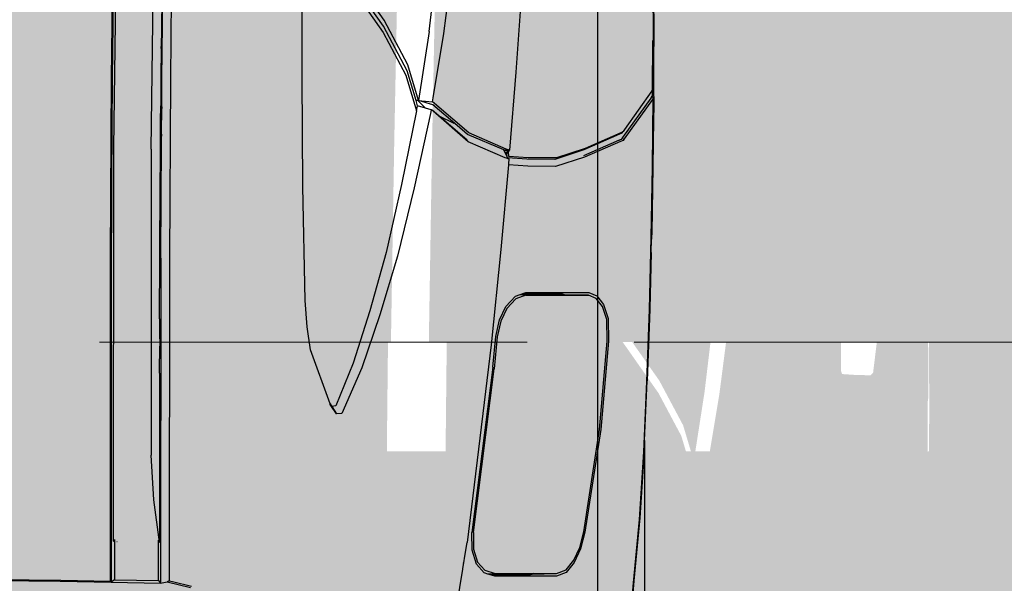
# Model space of a CAD drawing. Units: inches. Extents: x 1884 to 2398, y 474 to 1488.
# Tile 9 of 39: x 2247 to 2275, y 604 to 620. Entities that reach past the tile are written whole.
import ezdxf

# ---------------------------------------------------------------- set-up
doc = ezdxf.new("R2010")
doc.units = ezdxf.units.IN
doc.header["$MEASUREMENT"] = 0
doc.linetypes.add('ACAD_ISO02W100', pattern=[15, 12, -3])
doc.layers.get('0').update_dxf_attribs({"color": 250})
for name, color, linetype, lineweight in [('A-ANNO-DIMS', 2, 'Continuous', 18), ('A-FLOR-OVHD', 8, 'ACAD_ISO02W100', 18), ('C-VEHI', 8, 'Continuous', 18)]:
    doc.layers.add(name, color=color, linetype=linetype, lineweight=lineweight)
doc.layers.add('Edges', color=250, linetype='Continuous')
doc.layers.add('L-PVMT-PATT', color=9, linetype='Continuous', lineweight=13, true_color=0xc7c8ca)
doc.styles.get("Standard").update_dxf_attribs({"font": 'arial.ttf'})
doc.dimstyles.get("Standard").update_dxf_attribs({"dimtxt": 7, "dimasz": 0.18, "dimexe": 0.18, "dimexo": 0.0625, "dimgap": 0.09, "dimtad": 0, "dimtih": 1, "dimtoh": 1, "dimzin": 0, "dimdsep": 46, "dimlunit": 3, "dimtxsty": 'Standard', "dimcen": 0.09, "dimadec": 0, "dimazin": 0, "dimtfac": 1, "dimtofl": 0, "dimtmove": 0, "dimatfit": 3, "dimfxl": 1, "dimtolj": 1, "dimtzin": 0, "dimarcsym": 0})

# ---------------------------------------------------------------- blocks, each defined once
blk = doc.blocks.new('Nissan Qashqai pl')
at = {"layer": 'Edges'}
for p, q in [((10.61514, 12.81589), (10.66445, 12.81615)), ((10.61756, 12.81643), (10.66511, 12.81673)), ((10.66445, 12.81615), (10.7078, 12.81595)), ((10.66511, 12.81673), (10.66601, 12.81673)), ((10.66601, 12.81673), (10.67702, 12.8167)), ((10.67289, 12.81571), (10.70817, 12.81563)), ((10.68094, 12.81673), (10.67702, 12.8167)), ((10.71276, 12.81662), (10.68094, 12.81673)), ((10.7078, 12.81595), (10.70826, 12.81563)), ((10.70817, 12.81563), (10.7078, 12.81595)), ((10.70855, 12.81529), (10.70817, 12.81563)), ((10.70817, 12.81563), (10.70826, 12.81563)), ((10.70826, 12.81563), (10.70875, 12.81529)), ((10.70826, 12.81563), (10.71254, 12.81562)), ((10.70875, 12.81529), (10.7363, 12.79586)), ((10.71391, 12.81637), (10.71254, 12.81562)), ((10.71373, 12.81477), (10.71254, 12.81562)), ((10.71276, 12.81662), (10.76246, 12.8161)), ((10.71276, 12.81662), (10.72402, 12.81662)), ((10.71373, 12.81477), (10.71377, 12.81474)), ((10.74185, 12.79469), (10.71377, 12.81474)), ((10.71391, 12.81637), (10.7148, 12.81574)), ((10.76281, 12.81584), (10.71391, 12.81637)), ((10.7148, 12.81574), (10.74291, 12.79564)), ((10.76848, 12.8161), (10.72402, 12.81662)), ((10.76246, 12.8161), (10.76281, 12.8161)), ((10.76281, 12.8161), (10.80986, 12.81522)), ((10.81307, 12.81492), (10.76281, 12.81584)), ((10.76883, 12.8161), (10.76848, 12.8161)), ((10.80986, 12.81522), (10.76883, 12.8161)), ((10.80986, 12.81522), (10.81313, 12.81516)), ((10.86443, 12.81355), (10.81307, 12.81492)), ((10.81337, 12.81516), (10.81313, 12.81516)), ((10.81337, 12.81516), (10.81418, 12.81516)), ((10.81418, 12.81516), (10.81424, 12.81516)), ((10.82367, 12.81488), (10.81424, 12.81516)), ((10.82367, 12.81488), (10.86395, 12.8138)), ((10.85956, 12.81381), (10.85889, 12.81383)), ((10.86421, 12.81363), (10.85956, 12.81381)), ((10.86395, 12.8138), (10.8642, 12.81379)), ((10.8642, 12.81379), (10.91525, 12.81203)), ((10.91576, 12.81179), (10.86443, 12.81355)), ((10.95774, 12.81008), (10.91525, 12.81203)), ((10.9657, 12.8095), (10.91576, 12.81179)), ((10.95774, 12.81008), (10.9649, 12.80975)), ((10.95774, 12.81008), (11.12826, 12.81008)), ((10.9649, 12.80975), (11.01272, 12.8067)), ((11.01381, 12.80644), (10.9657, 12.8095)), ((11.01272, 12.8067), (11.05762, 12.80257)), ((11.05899, 12.80228), (11.01381, 12.80644)), ((11.05762, 12.80257), (11.07977, 12.80077)), ((11.07681, 12.80079), (11.05899, 12.80228)), ((10.7363, 12.79586), (10.73758, 12.79499)), ((10.73869, 12.794), (10.73758, 12.79499)), ((10.73758, 12.79499), (10.73776, 12.79462)), ((10.73776, 12.79462), (10.73792, 12.79451)), ((10.73776, 12.79462), (10.73846, 12.79316)), ((10.73846, 12.79316), (10.74965, 12.76789)), ((10.73869, 12.794), (10.73956, 12.79223)), ((10.73956, 12.79223), (10.7507, 12.76687)), ((10.74298, 12.79387), (10.74185, 12.79469)), ((10.74324, 12.79539), (10.74265, 12.7954)), ((10.74291, 12.79564), (10.74324, 12.79539)), ((10.74336, 12.79302), (10.74298, 12.79387)), ((10.74408, 12.79539), (10.74324, 12.79539)), ((10.74324, 12.79539), (10.74404, 12.7948)), ((10.74374, 12.79215), (10.74336, 12.79302)), ((10.74376, 12.7921), (10.74374, 12.79215)), ((10.74376, 12.7921), (10.75486, 12.76658)), ((10.74404, 12.7948), (10.74477, 12.79302)), ((10.74477, 12.79302), (10.75592, 12.76744)), ((10.86074, 12.78081), (10.87075, 12.78409)), ((10.87075, 12.78409), (10.88688, 12.78445)), ((10.88703, 12.78354), (10.87156, 12.78319)), ((10.88688, 12.78445), (10.94987, 12.77894)), ((10.94977, 12.77808), (10.88703, 12.78354)), ((10.85458, 12.77617), (10.86074, 12.78081)), ((10.86225, 12.78009), (10.85648, 12.77573)), ((10.87156, 12.78319), (10.86225, 12.78009)), ((11.02261, 12.76681), (10.94977, 12.77808)), ((10.94987, 12.77894), (11.02295, 12.7676)), ((10.85228, 12.77036), (10.85458, 12.77617)), ((10.85228, 12.72552), (10.85228, 12.77036)), ((10.85427, 12.77015), (10.85384, 12.753)), ((10.85648, 12.77573), (10.85427, 12.77015)), ((10.85427, 12.72549), (10.85427, 12.77015)), ((10.74965, 12.76789), (10.75648, 12.74726)), ((10.7507, 12.76687), (10.75747, 12.74624)), ((10.75592, 12.76744), (10.76258, 12.74675)), ((11.03387, 12.76392), (11.02261, 12.76681)), ((11.02295, 12.7676), (11.03477, 12.76454)), ((11.04293, 12.75972), (11.03387, 12.76392)), ((11.03477, 12.76454), (11.04442, 12.76006)), ((11.04973, 12.75421), (11.04293, 12.75972)), ((11.04442, 12.76006), (11.05161, 12.75423)), ((10.85278, 12.75031), (10.85348, 12.75208)), ((10.85278, 12.74201), (10.85278, 12.75031)), ((10.85348, 12.75208), (10.85384, 12.753)), ((10.85382, 12.75208), (10.85348, 12.75208)), ((10.85382, 12.75208), (10.85377, 12.75021)), ((10.85377, 12.75021), (10.85377, 12.74202)), ((10.85384, 12.753), (10.85382, 12.75208)), ((11.05232, 12.74746), (11.04973, 12.75421)), ((11.05161, 12.75423), (11.0543, 12.74726)), ((10.75648, 12.74726), (10.75627, 12.72726)), ((10.75747, 12.74624), (10.75723, 12.72633)), ((10.76258, 12.74675), (10.76229, 12.72686)), ((10.85278, 12.74201), (10.85377, 12.74202)), ((10.85278, 12.74194), (10.85278, 12.74201)), ((10.85377, 12.74194), (10.85278, 12.74194)), ((10.85278, 12.72416), (10.85278, 12.74194)), ((10.85377, 12.74202), (10.85377, 12.74194)), ((10.85377, 12.72143), (10.85377, 12.74194)), ((11.05275, 12.73004), (11.05232, 12.74746)), ((11.05232, 12.73118), (11.05232, 12.74746)), ((11.0543, 12.74726), (11.0543, 12.70347)), ((10.75627, 12.72726), (10.75535, 12.71342)), ((11.05231, 12.72872), (11.05232, 12.73118)), ((11.05282, 12.72741), (11.05231, 12.72872)), ((11.05231, 12.70374), (11.05231, 12.72872)), ((11.05232, 12.73118), (11.05275, 12.73004)), ((11.05282, 12.72741), (11.05275, 12.73004)), ((11.05275, 12.73004), (11.05381, 12.72731)), ((11.05282, 12.72741), (11.05281, 12.69855)), ((11.05381, 12.72731), (11.0538, 12.70183)), ((10.63183, 12.72283), (10.69546, 12.71842)), ((10.75723, 12.72633), (10.75631, 12.71262)), ((10.76229, 12.72686), (10.76145, 12.71309)), ((10.85278, 12.72416), (10.85228, 12.72552)), ((10.85377, 12.72143), (10.85278, 12.72416)), ((10.85498, 12.71814), (10.85377, 12.72143)), ((10.85427, 12.72549), (10.85688, 12.71839)), ((10.69546, 12.71842), (10.75092, 12.71398)), ((10.75069, 12.71321), (10.75013, 12.71142)), ((10.75059, 12.71106), (10.75069, 12.71321)), ((10.75069, 12.71321), (10.75092, 12.71398)), ((10.75097, 12.71319), (10.75069, 12.71321)), ((10.75224, 12.71309), (10.75092, 12.71398)), ((10.75161, 12.71314), (10.75092, 12.71398)), ((10.75535, 12.71342), (10.75224, 12.71309)), ((10.75631, 12.71262), (10.75727, 12.71346)), ((10.75727, 12.71346), (10.75689, 12.71249)), ((10.75727, 12.71346), (10.76044, 12.71318)), ((10.76044, 12.71318), (10.76145, 12.71309)), ((10.8622, 12.71137), (10.85498, 12.71814)), ((10.85688, 12.71839), (10.86374, 12.71199)), ((10.75013, 12.71142), (10.73867, 12.68487)), ((10.75073, 12.70976), (10.73966, 12.68398)), ((10.75628, 12.71091), (10.74486, 12.68432)), ((10.75111, 12.71066), (10.75073, 12.70976)), ((10.75244, 12.71062), (10.75073, 12.70976)), ((10.75189, 12.7128), (10.75111, 12.71066)), ((10.75224, 12.71309), (10.75161, 12.71314)), ((10.75189, 12.7128), (10.75161, 12.71314)), ((10.75256, 12.71241), (10.75189, 12.7128)), ((10.75244, 12.71062), (10.75256, 12.71241)), ((10.75565, 12.71222), (10.75244, 12.71062)), ((10.75256, 12.71241), (10.75259, 12.71271)), ((10.75322, 12.71203), (10.75256, 12.71241)), ((10.75565, 12.71222), (10.75322, 12.71203)), ((10.75612, 12.71246), (10.75565, 12.71222)), ((10.75612, 12.71246), (10.75631, 12.71262)), ((10.75629, 12.71247), (10.75612, 12.71246)), ((10.75628, 12.71228), (10.75614, 12.71226)), ((10.75689, 12.71249), (10.75628, 12.71091)), ((10.75629, 12.71247), (10.75628, 12.71228)), ((10.75631, 12.71262), (10.75629, 12.71247)), ((10.75689, 12.71249), (10.75629, 12.71247)), ((10.76145, 12.71309), (10.82176, 12.70767)), ((10.82176, 12.70767), (10.88962, 12.70079)), ((10.87182, 12.70675), (10.8622, 12.71137)), ((10.86374, 12.71199), (10.87273, 12.70768)), ((10.8836, 12.70407), (10.87182, 12.70675)), ((10.87273, 12.70768), (10.88392, 12.7051)), ((10.90536, 12.702), (10.8836, 12.70407)), ((10.88392, 12.7051), (10.90668, 12.70291)), ((10.88962, 12.70079), (11.03041, 12.68383)), ((10.90536, 12.702), (11.02317, 12.68714)), ((11.02306, 12.68821), (10.90668, 12.70291)), ((11.05008, 12.69636), (11.05231, 12.70374)), ((11.0538, 12.70183), (11.05281, 12.69855)), ((11.0543, 12.70347), (11.0538, 12.70183)), ((11.04427, 12.69114), (11.05008, 12.69636)), ((11.05198, 12.69583), (11.0458, 12.69029)), ((11.05281, 12.69855), (11.05198, 12.69583)), ((11.02306, 12.68821), (11.03497, 12.68825)), ((11.03579, 12.68719), (11.02317, 12.68714)), ((11.03497, 12.68825), (11.04427, 12.69114)), ((11.0458, 12.69029), (11.03579, 12.68719)), ((10.73867, 12.68487), (10.71766, 12.66037)), ((10.74486, 12.68432), (10.72325, 12.65939)), ((10.74379, 12.68361), (10.72652, 12.66353)), ((10.73966, 12.68398), (10.73336, 12.67661)), ((11.03575, 12.68287), (11.03041, 12.68383)), ((11.04905, 12.68071), (11.03575, 12.68287)), ((11.04495, 12.68119), (11.04481, 12.68121)), ((11.04919, 12.68069), (11.04905, 12.68071)), ((11.13359, 12.66697), (11.04919, 12.68069)), ((10.6678, 12.66721), (10.61519, 12.67398)), ((10.73336, 12.67661), (10.71859, 12.65933)), ((10.72652, 12.66353), (10.73162, 12.67411)), ((10.71369, 12.65953), (10.6678, 12.66721)), ((10.66642, 12.65663), (10.61435, 12.66285)), ((10.71653, 12.65907), (10.71369, 12.65953)), ((10.71859, 12.65933), (10.71545, 12.64901)), ((10.71545, 12.64901), (10.71653, 12.65907)), ((10.71766, 12.66037), (10.71653, 12.65907)), ((10.7221, 12.65809), (10.72089, 12.65399)), ((10.72325, 12.65939), (10.7221, 12.65809)), ((10.7221, 12.65809), (10.72238, 12.65871)), ((10.7221, 12.65809), (10.72473, 12.6575)), ((10.72652, 12.66353), (10.72238, 12.65871)), ((10.72473, 12.6575), (10.77763, 12.64599)), ((10.66642, 12.65663), (10.71545, 12.64901)), ((10.72089, 12.65399), (10.71545, 12.64846)), ((10.72089, 12.65399), (10.71925, 12.64842)), ((10.71545, 12.64901), (10.69003, 12.64139)), ((10.71545, 12.64729), (10.6943, 12.64099)), ((10.69755, 12.64007), (10.72279, 12.64766)), ((10.71545, 12.64901), (10.71545, 12.64846)), ((10.71545, 12.64846), (10.71545, 12.64729)), ((10.71925, 12.64842), (10.71545, 12.64729)), ((10.72279, 12.64766), (10.71925, 12.64842)), ((10.72279, 12.64766), (10.77536, 12.63703)), ((10.77763, 12.64599), (10.82645, 12.63413)), ((10.69003, 12.64139), (10.65826, 12.62446)), ((10.6943, 12.64099), (10.6627, 12.62415)), ((10.6671, 12.62384), (10.69755, 12.64007)), ((10.77536, 12.63703), (10.82385, 12.62606)), ((10.82645, 12.63413), (10.86821, 12.62158)), ((10.65826, 12.62446), (10.62146, 12.59859)), ((10.6627, 12.62415), (10.62607, 12.5984)), ((10.63062, 12.59823), (10.6671, 12.62384)), ((10.82385, 12.62606), (10.86528, 12.61443)), ((10.86821, 12.62158), (10.90591, 12.60869)), ((10.86528, 12.61443), (10.90264, 12.60247)), ((10.90591, 12.60869), (10.9384, 12.5945)), ((10.90264, 12.60247), (10.93299, 12.59007)), ((10.9384, 12.5945), (10.93862, 12.59051)), ((10.93159, 12.58602), (10.93344, 12.5872)), ((10.93345, 12.58712), (10.932, 12.58617)), ((10.93299, 12.59007), (10.93344, 12.5872)), ((10.93344, 12.5872), (10.93862, 12.59051)), ((10.93344, 12.5872), (10.93345, 12.58712)), ((10.93862, 12.59051), (10.93345, 12.58712)), ((10.93159, 12.58602), (10.89318, 12.57197)), ((10.932, 12.58617), (10.93159, 12.58602)), ((10.69879, 12.56623), (10.58925, 12.56589)), ((10.77686, 12.56674), (10.69879, 12.56623)), ((10.85804, 12.56829), (10.77686, 12.56674)), ((10.87661, 12.56967), (10.85804, 12.56829)), ((10.89318, 12.57197), (10.87661, 12.56967)), ((11.05807, 12.47379), (11.06139, 12.48725)), ((11.05822, 12.46998), (11.06236, 12.48656)), ((10.69998, 12.46617), (10.55662, 12.46771)), ((10.55723, 12.47372), (10.7004, 12.47221)), ((10.7004, 12.47221), (10.82794, 12.47151)), ((10.82794, 12.47151), (11.05437, 12.47137)), ((11.05437, 12.47137), (11.05754, 12.47139)), ((11.05754, 12.47139), (11.05807, 12.47379)), ((11.05754, 12.47139), (11.05822, 12.46998)), ((11.05921, 12.4653), (11.05822, 12.46998)), ((10.55757, 12.46751), (10.6649, 12.46591)), ((10.58658, 12.46697), (10.6649, 12.46591)), ((10.6649, 12.46591), (10.67863, 12.46575)), ((10.6649, 12.46591), (10.67717, 12.46572)), ((10.67863, 12.4657), (10.67717, 12.46572)), ((10.67863, 12.46575), (10.67863, 12.46616)), ((10.67863, 12.4657), (10.67863, 12.46575)), ((10.67863, 12.46575), (10.68008, 12.46573)), ((10.67863, 12.4657), (10.68008, 12.46568)), ((10.68008, 12.46616), (10.68008, 12.46573)), ((10.68008, 12.46573), (10.68008, 12.46568)), ((10.68008, 12.46573), (10.68111, 12.46572)), ((10.68008, 12.46568), (10.68111, 12.46566)), ((10.68111, 12.46616), (10.68111, 12.46572)), ((10.68111, 12.46572), (10.68111, 12.46566)), ((10.68111, 12.46572), (10.69913, 12.46552)), ((10.68111, 12.46566), (10.69658, 12.46543)), ((10.68111, 12.46566), (10.69913, 12.46552)), ((10.69658, 12.46543), (10.71439, 12.46535)), ((10.69913, 12.46552), (10.71439, 12.46535)), ((10.7201, 12.46605), (10.69998, 12.46617)), ((10.71439, 12.46535), (10.72388, 12.46529)), ((10.7201, 12.46605), (10.73056, 12.46525)), ((10.73952, 12.46594), (10.7201, 12.46605)), ((10.72388, 12.46529), (10.72479, 12.46525)), ((10.73056, 12.46525), (10.72479, 12.46525)), ((10.73114, 12.46521), (10.73056, 12.46525)), ((10.74955, 12.46515), (10.73114, 12.46521)), ((10.73114, 12.46521), (10.75016, 12.46511)), ((10.73952, 12.46594), (10.74955, 12.46515)), ((10.79225, 12.46563), (10.73952, 12.46594)), ((10.81792, 12.46479), (10.74955, 12.46515)), ((10.75016, 12.46511), (10.75041, 12.46509)), ((10.75041, 12.46509), (10.78083, 12.46489)), ((10.78083, 12.46489), (10.81792, 12.46479)), ((10.79225, 12.46519), (10.79225, 12.46563)), ((10.79328, 12.46563), (10.79225, 12.46563)), ((10.79328, 12.46519), (10.79328, 12.46563)), ((10.80401, 12.46556), (10.79328, 12.46563)), ((10.80401, 12.46527), (10.80401, 12.46556)), ((10.80748, 12.46554), (10.80401, 12.46556)), ((10.80748, 12.46554), (10.80748, 12.46529)), ((10.811, 12.46552), (10.80748, 12.46554)), ((10.811, 12.46552), (10.811, 12.46531)), ((10.81447, 12.4655), (10.811, 12.46552)), ((10.81447, 12.46534), (10.81447, 12.4655)), ((10.82786, 12.46543), (10.81447, 12.4655)), ((10.82767, 12.46474), (10.81792, 12.46479)), ((10.8711, 12.4646), (10.82767, 12.46474)), ((10.82786, 12.46543), (11.05921, 12.4653)), ((10.8711, 12.4646), (10.88236, 12.46459)), ((10.88236, 12.46459), (10.88251, 12.46459)), ((10.88251, 12.46459), (10.88837, 12.46461)), ((10.88837, 12.46461), (10.89229, 12.46458)), ((10.89229, 12.46458), (10.89957, 12.46459)), ((10.90974, 12.46456), (10.89957, 12.46459)), ((10.90974, 12.46456), (10.93988, 12.46456)), ((10.93988, 12.46456), (10.9491, 12.46453)), ((10.9491, 12.46453), (11.03007, 12.46452)), ((11.03007, 12.46452), (10.99996, 12.46051)), ((11.03005, 12.46373), (11.02866, 12.46373)), ((11.03005, 12.46351), (11.03005, 12.46373)), ((11.05743, 12.46372), (11.03005, 12.46373)), ((11.03006, 12.4642), (11.03007, 12.46452)), ((11.05683, 12.43232), (11.05743, 12.46372)), ((11.05743, 12.46372), (11.05921, 12.4653)), ((11.05854, 12.42997), (11.05921, 12.4653)), ((10.75022, 12.45862), (10.62366, 12.46028)), ((10.75022, 12.45862), (10.96805, 12.45851)), ((10.99996, 12.46051), (10.96805, 12.45851)), ((10.62233, 12.43331), (10.7493, 12.43163)), ((11.02948, 12.43407), (11.02949, 12.43429)), ((10.55607, 12.43229), (10.69961, 12.43079)), ((10.69989, 12.43035), (10.5563, 12.43184)), ((10.69961, 12.43079), (10.77221, 12.43038)), ((10.82704, 12.42966), (10.69989, 12.43035)), ((10.7493, 12.43163), (11.02943, 12.43154)), ((10.77221, 12.43038), (10.77221, 12.4302)), ((10.77221, 12.43038), (10.78885, 12.43029)), ((10.78885, 12.43016), (10.78885, 12.43029)), ((10.78885, 12.43029), (10.79225, 12.43027)), ((10.79225, 12.43015), (10.79225, 12.43027)), ((10.79225, 12.43027), (10.79328, 12.43026)), ((10.79328, 12.43015), (10.79328, 12.43026)), ((10.79328, 12.43026), (10.82673, 12.43008)), ((10.82673, 12.43008), (11.05854, 12.42997)), ((10.91328, 12.42962), (10.82704, 12.42966)), ((10.91328, 12.42962), (10.91328, 12.42978)), ((10.91374, 12.42962), (10.91328, 12.42962)), ((10.91374, 12.42962), (10.91378, 12.42978)), ((10.97147, 12.4296), (10.91374, 12.42962)), ((10.97151, 12.42986), (10.97147, 12.4296)), ((11.05789, 12.42956), (10.97147, 12.4296)), ((11.0281, 12.43233), (11.05683, 12.43232)), ((11.02943, 12.43154), (11.02944, 12.43164)), ((11.05683, 12.43232), (11.05854, 12.42997)), ((11.05722, 12.39425), (11.05789, 12.42956)), ((11.05785, 12.39378), (11.05854, 12.42997)), ((11.05789, 12.42956), (11.05854, 12.42997)), ((11.05596, 12.28512), (11.05722, 12.39425)), ((11.0566, 12.28486), (11.05785, 12.39378))]:
    blk.add_line(p, q, dxfattribs=at)
blk = doc.blocks.new('car')
blk.add_blockref('Nissan Qashqai pl', (-9.74328, -11.91512))
blk = doc.blocks.new('carr')
blk.add_blockref('car', (0.51244, -0.00696))
blk = doc.blocks.new('*D23')
at = {"layer": 'A-ANNO-DIMS', "color": 0, "lineweight": -2, "transparency": 16777216}
for p, q in [((2272.304, 752.812), (2298.291, 752.812)), ((2298.111, 752.632), (2298.111, 670.29)), ((2298.111, 580.529), (2298.111, 662.871)), ((2272.304, 580.349), (2298.291, 580.349))]:
    blk.add_line(p, q, dxfattribs=at)
at = {"layer": 'A-ANNO-DIMS', "color": 0, "lineweight": 100, "transparency": 16777216}
for points in [[(2298.081, 752.632), (2298.141, 752.632), (2298.111, 752.812)], [(2298.081, 580.529), (2298.141, 580.529), (2298.111, 580.349)]]:
    blk.add_solid(points, dxfattribs=at)
at = {"layer": 'Defpoints', "color": 0, "lineweight": 100, "transparency": 16777216}
for p in [(2272.242, 752.812), (2272.242, 580.349), (2298.111, 580.349)]:
    blk.add_point(p, dxfattribs=at)
at = {"layer": 'A-ANNO-DIMS', "color": 0, "transparency": 16777216, "insert": (2298.111, 666.58), "char_height": 7, "attachment_point": 5}
blk.add_mtext('\\A1;CAR 14\'-4 1/2" TYP.', dxfattribs=at)
blk = doc.blocks.new('*D44')
at = {"layer": 'A-ANNO-DIMS', "color": 0, "lineweight": -2, "transparency": 16777216}
for p, q in [((2209.755, 1247.822), (2209.755, 484.005)), ((2230.029, 1247.822), (2230.029, 484.005)), ((2209.935, 484.185), (2229.849, 484.185)), ((2230.029, 484.185), (2230.209, 484.185))]:
    blk.add_line(p, q, dxfattribs=at)
at = {"layer": 'A-ANNO-DIMS', "color": 0, "lineweight": 100, "transparency": 16777216}
for points in [[(2209.935, 484.215), (2209.935, 484.155), (2209.755, 484.185)], [(2229.849, 484.215), (2229.849, 484.155), (2230.029, 484.185)]]:
    blk.add_solid(points, dxfattribs=at)
at = {"layer": 'Defpoints', "color": 0, "lineweight": 100, "transparency": 16777216}
for p in [(2209.755, 1247.885), (2230.029, 1247.885), (2230.029, 484.185)]:
    blk.add_point(p, dxfattribs=at)
at = {"layer": 'A-ANNO-DIMS', "color": 0, "transparency": 16777216, "insert": (2247.429, 484.185), "char_height": 7, "attachment_point": 5}
blk.add_mtext('\\A1;1\'-8 1/2"', dxfattribs=at)
blk = doc.blocks.new('*D45')
at = {"layer": 'A-ANNO-DIMS', "color": 0, "lineweight": -2, "transparency": 16777216}
for p, q in [((2242.617, 1322.822), (2242.617, 484.005)), ((2263.617, 1322.822), (2263.617, 484.005)), ((2242.797, 484.185), (2244.052, 484.185)), ((2263.437, 484.185), (2262.181, 484.185))]:
    blk.add_line(p, q, dxfattribs=at)
at = {"layer": 'A-ANNO-DIMS', "color": 0, "lineweight": 100, "transparency": 16777216}
for points in [[(2242.797, 484.215), (2242.797, 484.155), (2242.617, 484.185)], [(2263.437, 484.215), (2263.437, 484.155), (2263.617, 484.185)]]:
    blk.add_solid(points, dxfattribs=at)
at = {"layer": 'Defpoints', "color": 0, "lineweight": 100, "transparency": 16777216}
for p in [(2242.617, 1322.885), (2263.617, 1322.885), (2263.617, 484.185)]:
    blk.add_point(p, dxfattribs=at)
at = {"layer": 'A-ANNO-DIMS', "color": 0, "transparency": 16777216, "insert": (2253.117, 484.185), "char_height": 7, "attachment_point": 5}
blk.add_mtext('\\A1;1\'-9"', dxfattribs=at)

msp = doc.modelspace()

# ---------------------------------------------------------------- hatches: boundary and pattern name
at = {"layer": 'L-PVMT-PATT'}
h = msp.add_hatch(color=256, dxfattribs=at)
h.dxf.hatch_style = 1
h.paths.add_polyline_path([(2387.529, 769.966), (2351.529, 769.966), (2238.447, 769.966), (2238.447, 762.15), (2238.447, 754.445), (2126.529, 754.445), (2126.529, 676.183), (2134.868, 676.183), (2142.673, 676.183), (2142.673, 646.578), (2134.868, 646.578), (2126.529, 646.578), (2126.529, 640.17), (2387.529, 640.17)])
h.paths.add_polyline_path([(2387.529, 631.385), (2303.086, 631.385), (2303.086, 615.671), (2387.529, 615.671)])
h.paths.add_polyline_path([(2387.529, 640.17), (2126.529, 640.17), (2126.529, 631.385), (2387.529, 631.385)])
h.paths.add_polyline_path([(2393.529, 604.13), (2387.529, 604.13), (2387.529, 615.671), (2303.086, 615.671), (2303.086, 607.943), (2249.649, 607.943), (2126.529, 607.943), (2126.529, 533.885), (2393.529, 533.885)])
h.paths.add_polyline_path([(2257.825, 611.008), (2257.83, 611.337), (2257.915, 616.493), (2258.021, 621.805), (2258.146, 627.274), (2258.252, 631.385), (2126.529, 631.385), (2126.529, 611.008)])
h.paths.add_polyline_path([(2258.892, 611.285), (2258.888, 611.008), (2300.247, 611.008), (2300.247, 631.385), (2259.314, 631.385), (2259.206, 627.173), (2259.081, 621.72), (2258.976, 616.424)])
h = msp.add_hatch(color=256, dxfattribs=at)
h.dxf.hatch_style = 1
h.paths.add_polyline_path([(2216.015, 611.008), (2212.351, 611.008), (2212.342, 608.327), (2212.34, 607.943), (2216.046, 607.943), (2216.044, 608.264)])
h.paths.add_polyline_path([(2212.351, 611.008), (2211.081, 611.008), (2210.074, 609.575), (2209.435, 608.376), (2209.305, 607.943), (2212.34, 607.943), (2212.342, 608.327)])
h.paths.add_polyline_path([(2257.742, 611.008), (2249.649, 611.008), (2217.664, 611.008), (2217.692, 608.284), (2217.694, 607.943), (2249.649, 607.943), (2257.712, 607.943), (2257.713, 608.284)])
h.paths.add_polyline_path([(2266.79, 611.008), (2264.592, 611.008), (2265.355, 609.923), (2266.022, 608.672), (2266.241, 607.943), (2266.364, 607.943), (2266.622, 609.602)])
h.paths.add_polyline_path([(2263.055, 611.008), (2259.39, 611.008), (2259.361, 608.264), (2259.359, 607.943), (2263.065, 607.943), (2263.063, 608.327)])
h.paths.add_polyline_path([(2265.331, 609.575), (2264.325, 611.008), (2263.055, 611.008), (2263.063, 608.327), (2263.065, 607.943), (2266.1, 607.943), (2265.97, 608.376)])
h.paths.add_polyline_path([(2272.885, 609.347), (2272.901, 609.457), (2272.902, 609.679), (2272.895, 611.008), (2271.456, 611.008), (2271.351, 610.147), (2271.277, 610.077), (2270.912, 610.081), (2270.481, 610.11), (2270.455, 610.183), (2270.448, 611.008), (2269.23, 611.008), (2269.228, 610.963), (2269.055, 608.458), (2269.014, 607.943), (2272.869, 607.943), (2272.882, 607.958)])
h.paths.add_polyline_path([(2269.228, 610.963), (2269.23, 611.008), (2267.227, 611.008), (2267.038, 609.547), (2266.77, 607.943), (2269.014, 607.943), (2269.055, 608.458)])
h.paths.add_polyline_path([(2293.178, 611.008), (2272.917, 611.008), (2272.925, 609.643), (2272.924, 609.184), (2272.925, 609.03), (2272.921, 607.943), (2293.123, 607.943), (2293.127, 608.565), (2293.159, 610.362)])
h.paths.add_polyline_path([(2302.932, 613.651), (2302.931, 615.98), (2302.91, 623.22), (2302.851, 630.905), (2302.844, 631.385), (2300.247, 631.385), (2300.247, 612.163), (2300.885, 611.925), (2301.121, 611.86), (2301.743, 612.576)])
h.paths.add_polyline_path([(2302.992, 610.861), (2302.993, 612.796), (2302.965, 612.8), (2301.576, 611.546), (2300.954, 610.83), (2300.899, 610.766), (2300.444, 610.894), (2300.139, 611.008), (2299.369, 611.008), (2299.448, 609.776), (2299.311, 611.008), (2299.207, 611.008), (2299.34, 609.722), (2299.553, 607.943), (2300.825, 607.943), (2300.851, 607.993), (2301.87, 609.442)])
h.paths.add_polyline_path([(2298.512, 611.008), (2296.882, 611.008), (2296.979, 609.034), (2297.054, 607.943), (2298.828, 607.943), (2298.736, 608.659)])
h.paths.add_polyline_path([(2294.51, 608.662), (2294.51, 608.662), (2294.362, 610.672), (2294.359, 611.008), (2293.338, 611.008), (2293.331, 610.606), (2293.329, 610.538), (2293.315, 609.691), (2293.305, 607.943), (2294.597, 607.943)])
h.paths.add_polyline_path([(2302.991, 609.68), (2301.718, 608.051), (2301.642, 607.943), (2302.986, 607.943)], flags=17)

# ---------------------------------------------------------------- linework, layer by layer
at = {"layer": 'A-FLOR-OVHD'}
msp.add_line((2249.649, 611.008), (2300.247, 611.008), dxfattribs=at)

# ---------------------------------------------------------------- block references
at = {"layer": 'C-VEHI', "xscale": 39.37007874015748, "yscale": 39.37007874015748, "zscale": 39.37007874015748, "rotation": 270}
msp.add_blockref('carr', (2229.977, 676.232), dxfattribs=at)

# ---------------------------------------------------------------- dimensions: what is measured, and where the dimension line sits
at = {"layer": 'A-ANNO-DIMS'}
for base, p1, p2, picture, middle in [((2263.617, 484.185), (2242.617, 1322.885), (2263.617, 1322.885), '*D45', (2253.117, 484.185)), ((2230.029, 484.185), (2209.755, 1247.885), (2230.029, 1247.885), '*D44', (2247.429, 484.185))]:
    dim = msp.add_linear_dim(base=base, p1=p1, p2=p2, dimstyle='Standard', override={"dimdec": 1, "dimlfac": 1, "dimrnd": 0, "dimzin": 1, "dimdsep": 46, "dimlunit": 4, "dimfrac": 2}, dxfattribs=at)
    dim.commit()
    dim.dimension.update_dxf_attribs({"geometry": picture, "text_midpoint": middle})
dim = msp.add_linear_dim(base=(2298.111, 580.349), p1=(2272.242, 752.812), p2=(2272.242, 580.349), angle=270, text='CAR <> TYP.', dimstyle='Standard', override={"dimdec": 1, "dimlfac": 1, "dimrnd": 0, "dimzin": 1, "dimdsep": 46, "dimlunit": 4, "dimfrac": 2}, dxfattribs=at)
dim.commit()
dim.dimension.update_dxf_attribs({"geometry": '*D23', "text_midpoint": (2298.111, 666.58)})

doc.saveas('drawing.dxf')
